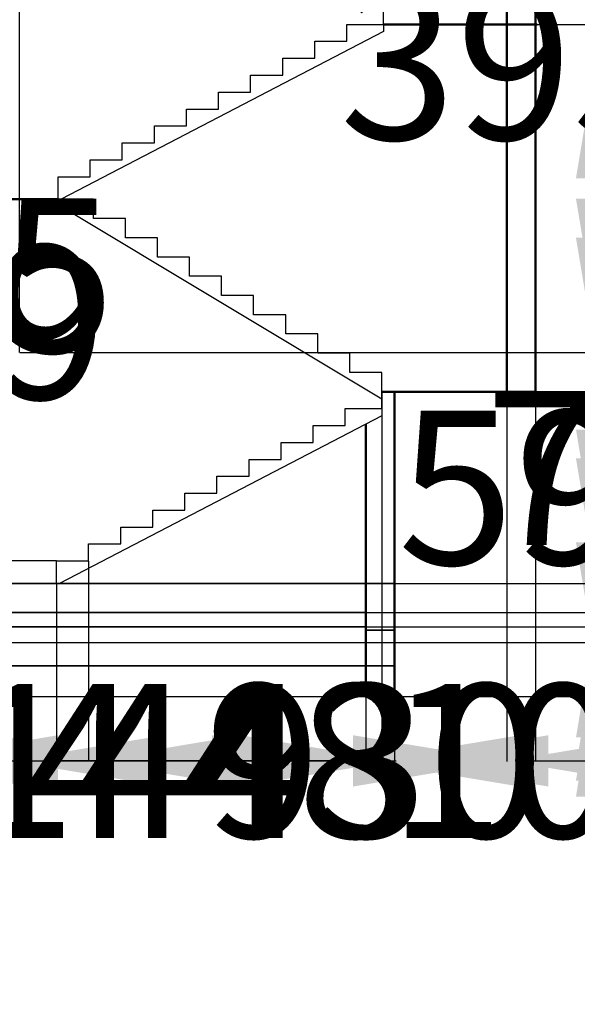
# Model space of a CAD drawing. Units: inches. Extents: x 131 to 858, y -65 to 554.
# Tile 2 of 4: x 431 to 605, y -65 to 242. Entities that reach past the tile are written whole.
import ezdxf

# ---------------------------------------------------------------- set-up
doc = ezdxf.new("R2010")
doc.units = ezdxf.units.IN
doc.header["$MEASUREMENT"] = 0
for name, color, linetype, lineweight in [('A-ANNO-DIMS', 2, 'Continuous', 18), ('A-FLOR-STRS', 3, 'Continuous', 25), ('A-SECT', 7, 'Continuous', 50), ('S-FNDN', 1, 'Continuous', 35)]:
    doc.layers.add(name, color=color, linetype=linetype, lineweight=lineweight)
doc.styles.get("Standard").update_dxf_attribs({"font": 'arial.ttf'})
doc.dimstyles.get("Standard").update_dxf_attribs({"dimtxt": 48, "dimasz": 48, "dimexe": 0.18, "dimexo": 0.0625, "dimgap": 0.09, "dimtad": 0, "dimtih": 1, "dimtoh": 1, "dimdec": 0, "dimrnd": 72, "dimzin": 0, "dimdsep": 46, "dimlunit": 3, "dimtxsty": 'Standard', "dimcen": 0.09, "dimadec": 0, "dimazin": 0, "dimtfac": 1, "dimtdec": 0, "dimtofl": 0, "dimtmove": 0, "dimatfit": 3, "dimfxl": 1, "dimtolj": 1, "dimtzin": 0, "dimarcsym": 0})

# ---------------------------------------------------------------- blocks, each defined once
blk = doc.blocks.new('*D8')
at = {"layer": 'A-ANNO-DIMS', "color": 0, "lineweight": -2, "transparency": 16777216}
for p, q in [((334.01, 66.49), (334.01, 11.06)), ((338.01, 66.49), (338.01, 11.06)), ((286.01, 11.24), (238.01, 11.24)), ((386.01, 11.24), (434.01, 11.24))]:
    blk.add_line(p, q, dxfattribs=at)
at = {"layer": 'A-ANNO-DIMS', "color": 0, "transparency": 16777216}
for points in [[(286.01, 19.24), (286.01, 3.24), (334.01, 11.24)], [(386.01, 19.24), (386.01, 3.24), (338.01, 11.24)]]:
    blk.add_solid(points, dxfattribs=at)
at = {"layer": 'Defpoints', "color": 0, "transparency": 16777216}
for p in [(334.01, 66.55), (338.01, 66.55), (338.01, 11.24)]:
    blk.add_point(p, dxfattribs=at)
at = {"layer": 'A-ANNO-DIMS', "color": 0, "transparency": 16777216, "insert": (450.7, 11.24), "char_height": 48, "attachment_point": 5}
blk.add_mtext('\\A1;4', dxfattribs=at)
blk = doc.blocks.new('*D9')
at = {"layer": 'A-ANNO-DIMS', "color": 0, "lineweight": -2, "transparency": 16777216}
for p, q in [((338.01, 66.49), (338.01, 11.06)), ((386.01, 31.27), (386.01, 11.06)), ((290.01, 11.24), (242.01, 11.24)), ((434.01, 11.24), (482.01, 11.24))]:
    blk.add_line(p, q, dxfattribs=at)
at = {"layer": 'A-ANNO-DIMS', "color": 0, "transparency": 16777216}
for points in [[(290.01, 19.24), (290.01, 3.24), (338.01, 11.24)], [(434.01, 19.24), (434.01, 3.24), (386.01, 11.24)]]:
    blk.add_solid(points, dxfattribs=at)
at = {"layer": 'Defpoints', "color": 0, "transparency": 16777216}
for p in [(338.01, 66.55), (386.01, 31.34), (386.01, 11.24)]:
    blk.add_point(p, dxfattribs=at)
at = {"layer": 'A-ANNO-DIMS', "color": 0, "transparency": 16777216, "insert": (517.5, 11.24), "char_height": 48, "attachment_point": 5}
blk.add_mtext('\\A1;48', dxfattribs=at)
blk = doc.blocks.new('*D10')
at = {"layer": 'A-ANNO-DIMS', "color": 0, "lineweight": -2, "transparency": 16777216}
for p, q in [((386.01, 31.27), (386.01, 11.06)), ((395.01, 31.27), (395.01, 11.06)), ((338.01, 11.24), (290.01, 11.24)), ((443.01, 11.24), (491.01, 11.24))]:
    blk.add_line(p, q, dxfattribs=at)
at = {"layer": 'A-ANNO-DIMS', "color": 0, "transparency": 16777216}
for points in [[(338.01, 19.24), (338.01, 3.24), (386.01, 11.24)], [(443.01, 19.24), (443.01, 3.24), (395.01, 11.24)]]:
    blk.add_solid(points, dxfattribs=at)
at = {"layer": 'Defpoints', "color": 0, "transparency": 16777216}
for p in [(386.01, 31.34), (395.01, 31.34), (395.01, 11.24)]:
    blk.add_point(p, dxfattribs=at)
at = {"layer": 'A-ANNO-DIMS', "color": 0, "transparency": 16777216, "insert": (506.89, 11.24), "char_height": 48, "attachment_point": 5}
blk.add_mtext('\\A1;9', dxfattribs=at)
blk = doc.blocks.new('*D11')
at = {"layer": 'A-ANNO-DIMS', "color": 0, "lineweight": -2, "transparency": 16777216}
for p, q in [((395.014446, 31.273524), (395.014446, 11.056024)), ((539.014446, 31.273524), (539.014446, 11.056024)), ((347.014446, 11.236024), (299.014446, 11.236024)), ((587.014446, 11.236024), (635.014446, 11.236024))]:
    blk.add_line(p, q, dxfattribs=at)
at = {"layer": 'A-ANNO-DIMS', "color": 0, "transparency": 16777216}
for points in [[(347.014446, 19.236024), (347.014446, 3.236024), (395.014446, 11.236024)], [(587.014446, 19.236024), (587.014446, 3.236024), (539.014446, 11.236024)]]:
    blk.add_solid(points, dxfattribs=at)
at = {"layer": 'Defpoints', "color": 0, "transparency": 16777216}
for p in [(395.014446, 31.336024), (539.014446, 31.336024), (539.014446, 11.236024)]:
    blk.add_point(p, dxfattribs=at)
at = {"layer": 'A-ANNO-DIMS', "color": 0, "transparency": 16777216, "insert": (467.014446, 11.236024), "char_height": 48, "attachment_point": 5}
blk.add_mtext('\\A1;144', dxfattribs=at)
blk = doc.blocks.new('*D12')
at = {"layer": 'A-ANNO-DIMS', "color": 0, "lineweight": -2, "transparency": 16777216}
for p, q in [((539.01, 31.27), (539.01, 11.06)), ((548.01, 31.27), (548.01, 11.06)), ((491.01, 11.24), (443.01, 11.24)), ((596.01, 11.24), (644.01, 11.24))]:
    blk.add_line(p, q, dxfattribs=at)
at = {"layer": 'A-ANNO-DIMS', "color": 0, "transparency": 16777216}
for points in [[(491.01, 19.24), (491.01, 3.24), (539.01, 11.24)], [(596.01, 19.24), (596.01, 3.24), (548.01, 11.24)]]:
    blk.add_solid(points, dxfattribs=at)
at = {"layer": 'Defpoints', "color": 0, "transparency": 16777216}
for p in [(539.01, 31.34), (548.01, 31.34), (548.01, 11.24)]:
    blk.add_point(p, dxfattribs=at)
at = {"layer": 'A-ANNO-DIMS', "color": 0, "transparency": 16777216, "insert": (659.89, 11.24), "char_height": 48, "attachment_point": 5}
blk.add_mtext('\\A1;9', dxfattribs=at)
blk = doc.blocks.new('*D13')
at = {"layer": 'A-ANNO-DIMS', "color": 0, "lineweight": -2, "transparency": 16777216}
for p, q in [((592.04, 126.29), (592.04, 11.06)), ((548.01, 31.27), (548.01, 11.06)), ((500.01, 11.24), (452.01, 11.24)), ((640.04, 11.24), (688.04, 11.24))]:
    blk.add_line(p, q, dxfattribs=at)
at = {"layer": 'A-ANNO-DIMS', "color": 0, "transparency": 16777216}
for points in [[(500.01, 19.24), (500.01, 3.24), (548.01, 11.24)], [(640.04, 19.24), (640.04, 3.24), (592.04, 11.24)]]:
    blk.add_solid(points, dxfattribs=at)
at = {"layer": 'Defpoints', "color": 0, "transparency": 16777216}
for p in [(592.04, 126.36), (548.01, 31.34), (592.04, 11.24)]:
    blk.add_point(p, dxfattribs=at)
at = {"layer": 'A-ANNO-DIMS', "color": 0, "transparency": 16777216, "insert": (770.09, 11.24), "char_height": 48, "attachment_point": 5}
blk.add_mtext('\\A1;44.03', dxfattribs=at)
blk = doc.blocks.new('*D14')
at = {"layer": 'A-ANNO-DIMS', "color": 0, "lineweight": -2, "transparency": 16777216}
for p, q in [((592.11, 426.55), (612.82, 426.55)), ((612.64, 378.55), (612.64, 253.56)), ((612.64, 79.34), (612.64, 204.33)), ((233.08, 31.34), (612.82, 31.34))]:
    blk.add_line(p, q, dxfattribs=at)
at = {"layer": 'A-ANNO-DIMS', "color": 0, "transparency": 16777216}
for points in [[(604.64, 378.55), (620.64, 378.55), (612.64, 426.55)], [(604.64, 79.34), (620.64, 79.34), (612.64, 31.34)]]:
    blk.add_solid(points, dxfattribs=at)
at = {"layer": 'Defpoints', "color": 0, "transparency": 16777216}
for p in [(592.04, 426.55), (612.64, 426.55), (233.01, 31.34)]:
    blk.add_point(p, dxfattribs=at)
at = {"layer": 'A-ANNO-DIMS', "color": 0, "transparency": 16777216, "insert": (612.64, 228.94), "char_height": 48, "attachment_point": 5}
blk.add_mtext('\\A1;395.2', dxfattribs=at)
blk = doc.blocks.new('*D15')
at = {"layer": 'A-ANNO-DIMS', "color": 0, "lineweight": -2, "transparency": 16777216}
for p, q in [((212.91, 114.55), (212.91, 162.55)), ((212.91, 162.55), (260.91, 162.55)), ((385.95, 66.55), (212.73, 66.55)), ((385.95, 31.34), (212.73, 31.34)), ((212.91, -16.66), (212.91, -64.66))]:
    blk.add_line(p, q, dxfattribs=at)
at = {"layer": 'A-ANNO-DIMS', "color": 0, "transparency": 16777216}
for points in [[(204.91, 114.55), (220.91, 114.55), (212.91, 66.55)], [(204.91, -16.66), (220.91, -16.66), (212.91, 31.34)]]:
    blk.add_solid(points, dxfattribs=at)
at = {"layer": 'Defpoints', "color": 0, "transparency": 16777216}
for p in [(212.91, 66.55), (386.01, 66.55), (386.01, 31.34)]:
    blk.add_point(p, dxfattribs=at)
at = {"layer": 'A-ANNO-DIMS', "color": 0, "transparency": 16777216, "insert": (360.8, 162.55), "char_height": 48, "attachment_point": 5}
blk.add_mtext('\\A1;35.215', dxfattribs=at)
blk = doc.blocks.new('*D17')
at = {"layer": 'A-ANNO-DIMS', "color": 0, "lineweight": -2, "transparency": 16777216}
for p, q in [((212.91, 100.02), (212.91, 148.02)), ((212.91, 148.02), (260.91, 148.02)), ((232.95, 52.02), (212.73, 52.02)), ((232.95, 40.9), (212.73, 40.9)), ((212.91, -7.1), (212.91, -55.1))]:
    blk.add_line(p, q, dxfattribs=at)
at = {"layer": 'A-ANNO-DIMS', "color": 0, "transparency": 16777216}
for points in [[(204.91, 100.02), (220.91, 100.02), (212.91, 52.02)], [(204.91, -7.1), (220.91, -7.1), (212.91, 40.9)]]:
    blk.add_solid(points, dxfattribs=at)
at = {"layer": 'Defpoints', "color": 0, "transparency": 16777216}
for p in [(212.91, 52.02), (233.01, 52.02), (233.01, 40.9)]:
    blk.add_point(p, dxfattribs=at)
at = {"layer": 'A-ANNO-DIMS', "color": 0, "transparency": 16777216, "insert": (358.43, 148.02), "char_height": 48, "attachment_point": 5}
blk.add_mtext('\\A1;11.119', dxfattribs=at)
blk = doc.blocks.new('*D19')
at = {"layer": 'A-ANNO-DIMS', "color": 0, "lineweight": -2, "transparency": 16777216}
for p, q in [((612.64, 105.55), (612.64, 153.55)), ((612.64, 153.55), (660.64, 153.55)), ((242.08, 57.55), (612.82, 57.55)), ((242.08, 53.09), (612.82, 53.09)), ((612.64, 5.09), (612.64, -42.91))]:
    blk.add_line(p, q, dxfattribs=at)
at = {"layer": 'A-ANNO-DIMS', "color": 0, "transparency": 16777216}
for points in [[(604.64, 105.55), (620.64, 105.55), (612.64, 57.55)], [(604.64, 5.09), (620.64, 5.09), (612.64, 53.09)]]:
    blk.add_solid(points, dxfattribs=at)
at = {"layer": 'Defpoints', "color": 0, "transparency": 16777216}
for p in [(242.01, 57.55), (612.64, 57.55), (242.01, 53.09)]:
    blk.add_point(p, dxfattribs=at)
at = {"layer": 'A-ANNO-DIMS', "color": 0, "transparency": 16777216, "insert": (742.86, 153.55), "char_height": 48, "attachment_point": 5}
blk.add_mtext('\\A1;4.465', dxfattribs=at)
blk = doc.blocks.new('*D20')
at = {"layer": 'A-ANNO-DIMS', "color": 0, "lineweight": -2, "transparency": 16777216}
for p, q in [((612.64, 114.55), (612.64, 162.55)), ((612.64, 162.55), (660.64, 162.55)), ((242.08, 66.55), (612.82, 66.55)), ((242.08, 57.55), (612.82, 57.55)), ((612.64, 9.55), (612.64, -38.45))]:
    blk.add_line(p, q, dxfattribs=at)
at = {"layer": 'A-ANNO-DIMS', "color": 0, "transparency": 16777216}
for points in [[(604.64, 114.55), (620.64, 114.55), (612.64, 66.55)], [(604.64, 9.55), (620.64, 9.55), (612.64, 57.55)]]:
    blk.add_solid(points, dxfattribs=at)
at = {"layer": 'Defpoints', "color": 0, "transparency": 16777216}
for p in [(242.01, 66.55), (612.64, 66.55), (242.01, 57.55)]:
    blk.add_point(p, dxfattribs=at)
at = {"layer": 'A-ANNO-DIMS', "color": 0, "transparency": 16777216, "insert": (676.51, 162.55), "char_height": 48, "attachment_point": 5}
blk.add_mtext('\\A1;9', dxfattribs=at)
blk = doc.blocks.new('*D22')
at = {"layer": 'A-ANNO-DIMS', "color": 0, "lineweight": -2, "transparency": 16777216}
for p, q in [((612.64, 114.55), (612.64, 162.55)), ((612.64, 162.55), (660.64, 162.55)), ((395.08, 66.55), (612.82, 66.55)), ((395.08, 48.13), (612.82, 48.13)), ((612.64, 0.13), (612.64, -47.87))]:
    blk.add_line(p, q, dxfattribs=at)
at = {"layer": 'A-ANNO-DIMS', "color": 0, "transparency": 16777216}
for points in [[(604.64, 114.55), (620.64, 114.55), (612.64, 66.55)], [(604.64, 0.13), (620.64, 0.13), (612.64, 48.13)]]:
    blk.add_solid(points, dxfattribs=at)
at = {"layer": 'Defpoints', "color": 0, "transparency": 16777216}
for p in [(395.01, 66.55), (612.64, 66.55), (395.01, 48.13)]:
    blk.add_point(p, dxfattribs=at)
at = {"layer": 'A-ANNO-DIMS', "color": 0, "transparency": 16777216, "insert": (758.11, 162.55), "char_height": 48, "attachment_point": 5}
blk.add_mtext('\\A1;18.417', dxfattribs=at)
blk = doc.blocks.new('*D32')
at = {"layer": 'A-ANNO-DIMS', "color": 0, "lineweight": -2, "transparency": 16777216}
for p, q in [((347.01, 446.65), (299.01, 446.65)), ((395.01, 138.61), (395.01, 446.83)), ((431.01, 138.61), (431.01, 446.83)), ((479.01, 446.65), (527.01, 446.65))]:
    blk.add_line(p, q, dxfattribs=at)
at = {"layer": 'A-ANNO-DIMS', "color": 0, "transparency": 16777216}
for points in [[(347.01, 454.65), (347.01, 438.65), (395.01, 446.65)], [(479.01, 454.65), (479.01, 438.65), (431.01, 446.65)]]:
    blk.add_solid(points, dxfattribs=at)
at = {"layer": 'Defpoints', "color": 0, "transparency": 16777216}
for p in [(431.01, 446.65), (395.01, 138.55), (431.01, 138.55)]:
    blk.add_point(p, dxfattribs=at)
at = {"layer": 'A-ANNO-DIMS', "color": 0, "transparency": 16777216, "insert": (561.45, 446.65), "char_height": 48, "attachment_point": 5}
blk.add_mtext('\\A1;36', dxfattribs=at)
blk = doc.blocks.new('*D33')
at = {"layer": 'A-ANNO-DIMS', "color": 0, "lineweight": -2, "transparency": 16777216}
for p, q in [((612.639956, 186.551418), (612.639956, 234.551418)), ((431.076946, 138.551418), (612.819956, 138.551418)), ((431.076946, 66.551418), (612.819956, 66.551418)), ((612.639956, 18.551418), (612.639956, -29.448582))]:
    blk.add_line(p, q, dxfattribs=at)
at = {"layer": 'A-ANNO-DIMS', "color": 0, "transparency": 16777216}
for points in [[(604.639956, 186.551418), (620.639956, 186.551418), (612.639956, 138.551418)], [(604.639956, 18.551418), (620.639956, 18.551418), (612.639956, 66.551418)]]:
    blk.add_solid(points, dxfattribs=at)
at = {"layer": 'Defpoints', "color": 0, "transparency": 16777216}
for p in [(431.014446, 138.551418), (612.639956, 138.551418), (431.014446, 66.551418)]:
    blk.add_point(p, dxfattribs=at)
at = {"layer": 'A-ANNO-DIMS', "color": 0, "transparency": 16777216, "insert": (612.639956, 102.551418), "char_height": 48, "attachment_point": 5}
blk.add_mtext('\\A1;72', dxfattribs=at)
blk = doc.blocks.new('*D34')
at = {"layer": 'A-ANNO-DIMS', "color": 0, "lineweight": -2, "transparency": 16777216}
for p, q in [((398.01, 66.49), (398.01, 11.06)), ((428.01, 66.49), (428.01, 11.06)), ((350.01, 11.24), (302.01, 11.24)), ((476.01, 11.24), (524.01, 11.24))]:
    blk.add_line(p, q, dxfattribs=at)
at = {"layer": 'A-ANNO-DIMS', "color": 0, "transparency": 16777216}
for points in [[(350.01, 19.24), (350.01, 3.24), (398.01, 11.24)], [(476.01, 19.24), (476.01, 3.24), (428.01, 11.24)]]:
    blk.add_solid(points, dxfattribs=at)
at = {"layer": 'Defpoints', "color": 0, "transparency": 16777216}
for p in [(398.01, 66.55), (428.01, 66.55), (428.01, 11.24)]:
    blk.add_point(p, dxfattribs=at)
at = {"layer": 'A-ANNO-DIMS', "color": 0, "transparency": 16777216, "insert": (558.39, 11.24), "char_height": 48, "attachment_point": 5}
blk.add_mtext('\\A1;30', dxfattribs=at)
blk = doc.blocks.new('*D36')
at = {"layer": 'A-ANNO-DIMS', "color": 0, "lineweight": -2, "transparency": 16777216}
for p, q in [((452.53, 73.54), (452.53, 11.06)), ((442.52, 66.49), (442.52, 11.06)), ((394.52, 11.24), (346.52, 11.24)), ((500.53, 11.24), (548.53, 11.24))]:
    blk.add_line(p, q, dxfattribs=at)
at = {"layer": 'A-ANNO-DIMS', "color": 0, "transparency": 16777216}
for points in [[(394.52, 19.24), (394.52, 3.24), (442.52, 11.24)], [(500.53, 19.24), (500.53, 3.24), (452.53, 11.24)]]:
    blk.add_solid(points, dxfattribs=at)
at = {"layer": 'Defpoints', "color": 0, "transparency": 16777216}
for p in [(452.53, 73.6), (442.52, 66.55), (452.53, 11.24)]:
    blk.add_point(p, dxfattribs=at)
at = {"layer": 'A-ANNO-DIMS', "color": 0, "transparency": 16777216, "insert": (646, 11.24), "char_height": 48, "attachment_point": 5}
blk.add_mtext('\\A1;10.013', dxfattribs=at)
blk = doc.blocks.new('*D37')
at = {"layer": 'A-ANNO-DIMS', "color": 0, "lineweight": -2, "transparency": 16777216}
for p, q in [((544.04, 126.29), (544.04, 11.06)), ((452.53, 73.54), (452.53, 11.06)), ((404.53, 11.24), (356.53, 11.24)), ((592.04, 11.24), (640.04, 11.24))]:
    blk.add_line(p, q, dxfattribs=at)
at = {"layer": 'A-ANNO-DIMS', "color": 0, "transparency": 16777216}
for points in [[(404.53, 19.24), (404.53, 3.24), (452.53, 11.24)], [(592.04, 19.24), (592.04, 3.24), (544.04, 11.24)]]:
    blk.add_solid(points, dxfattribs=at)
at = {"layer": 'Defpoints', "color": 0, "transparency": 16777216}
for p in [(544.04, 126.36), (452.53, 73.6), (544.04, 11.24)]:
    blk.add_point(p, dxfattribs=at)
at = {"layer": 'A-ANNO-DIMS', "color": 0, "transparency": 16777216, "insert": (716.49, 11.24), "char_height": 48, "attachment_point": 5}
blk.add_mtext('\\A1;91.51', dxfattribs=at)
blk = doc.blocks.new('*D38')
at = {"layer": 'A-ANNO-DIMS', "color": 0, "lineweight": -2, "transparency": 16777216}
for p, q in [((544.04, 126.29), (544.04, 11.06)), ((583.04, 126.29), (583.04, 11.06)), ((496.04, 11.24), (448.04, 11.24)), ((631.04, 11.24), (679.04, 11.24))]:
    blk.add_line(p, q, dxfattribs=at)
at = {"layer": 'A-ANNO-DIMS', "color": 0, "transparency": 16777216}
for points in [[(496.04, 19.24), (496.04, 3.24), (544.04, 11.24)], [(631.04, 19.24), (631.04, 3.24), (583.04, 11.24)]]:
    blk.add_solid(points, dxfattribs=at)
at = {"layer": 'Defpoints', "color": 0, "transparency": 16777216}
for p in [(544.04, 126.36), (583.04, 126.36), (583.04, 11.24)]:
    blk.add_point(p, dxfattribs=at)
at = {"layer": 'A-ANNO-DIMS', "color": 0, "transparency": 16777216, "insert": (713.55, 11.24), "char_height": 48, "attachment_point": 5}
blk.add_mtext('\\A1;39', dxfattribs=at)
blk = doc.blocks.new('*D39')
at = {"layer": 'A-ANNO-DIMS', "color": 0, "lineweight": -2, "transparency": 16777216}
for p, q in [((583.04, 126.29), (583.04, 11.06)), ((592.04, 126.29), (592.04, 11.06)), ((535.04, 11.24), (487.04, 11.24)), ((640.04, 11.24), (688.04, 11.24))]:
    blk.add_line(p, q, dxfattribs=at)
at = {"layer": 'A-ANNO-DIMS', "color": 0, "transparency": 16777216}
for points in [[(535.04, 19.24), (535.04, 3.24), (583.04, 11.24)], [(640.04, 19.24), (640.04, 3.24), (592.04, 11.24)]]:
    blk.add_solid(points, dxfattribs=at)
at = {"layer": 'Defpoints', "color": 0, "transparency": 16777216}
for p in [(583.04, 126.36), (592.04, 126.36), (592.04, 11.24)]:
    blk.add_point(p, dxfattribs=at)
at = {"layer": 'A-ANNO-DIMS', "color": 0, "transparency": 16777216, "insert": (703.92, 11.24), "char_height": 48, "attachment_point": 5}
blk.add_mtext('\\A1;9', dxfattribs=at)
blk = doc.blocks.new('*D40')
at = {"layer": 'A-ANNO-DIMS', "color": 0, "lineweight": -2, "transparency": 16777216}
for p, q in [((212.91, 121.6), (212.91, 169.6)), ((212.91, 169.6), (260.91, 169.6)), ((442.46, 73.6), (212.73, 73.6)), ((442.46, 66.55), (212.73, 66.55)), ((212.91, 18.55), (212.91, -29.45))]:
    blk.add_line(p, q, dxfattribs=at)
at = {"layer": 'A-ANNO-DIMS', "color": 0, "transparency": 16777216}
for points in [[(204.91, 121.6), (220.91, 121.6), (212.91, 73.6)], [(204.91, 18.55), (220.91, 18.55), (212.91, 66.55)]]:
    blk.add_solid(points, dxfattribs=at)
at = {"layer": 'Defpoints', "color": 0, "transparency": 16777216}
for p in [(212.91, 73.6), (442.52, 73.6), (442.52, 66.55)]:
    blk.add_point(p, dxfattribs=at)
at = {"layer": 'A-ANNO-DIMS', "color": 0, "transparency": 16777216, "insert": (323.33, 169.6), "char_height": 48, "attachment_point": 5}
blk.add_mtext('\\A1;7.05', dxfattribs=at)
blk = doc.blocks.new('*D41')
at = {"layer": 'A-ANNO-DIMS', "color": 0, "lineweight": -2, "transparency": 16777216}
for p, q in [((612.64, 174.36), (612.64, 222.36)), ((592.11, 126.36), (612.82, 126.36)), ((548.08, 66.55), (612.82, 66.55)), ((612.64, 18.55), (612.64, -29.45))]:
    blk.add_line(p, q, dxfattribs=at)
at = {"layer": 'A-ANNO-DIMS', "color": 0, "transparency": 16777216}
for points in [[(604.64, 174.36), (620.64, 174.36), (612.64, 126.36)], [(604.64, 18.55), (620.64, 18.55), (612.64, 66.55)]]:
    blk.add_solid(points, dxfattribs=at)
at = {"layer": 'Defpoints', "color": 0, "transparency": 16777216}
for p in [(592.04, 126.36), (612.64, 126.36), (548.01, 66.55)]:
    blk.add_point(p, dxfattribs=at)
at = {"layer": 'A-ANNO-DIMS', "color": 0, "transparency": 16777216, "insert": (612.64, 96.45), "char_height": 48, "attachment_point": 5}
blk.add_mtext('\\A1;59.8', dxfattribs=at)
blk = doc.blocks.new('*D42')
at = {"layer": 'A-ANNO-DIMS', "color": 0, "lineweight": -2, "transparency": 16777216}
for p, q in [((612.64, 240.89), (612.64, 288.89)), ((612.64, 288.89), (660.64, 288.89)), ((592.6, 240.89), (612.82, 240.89)), ((612.64, 174.36), (612.64, 192.89)), ((592.11, 126.36), (612.82, 126.36))]:
    blk.add_line(p, q, dxfattribs=at)
at = {"layer": 'A-ANNO-DIMS', "color": 0, "transparency": 16777216}
for points in [[(604.64, 192.89), (620.64, 192.89), (612.64, 240.89)], [(604.64, 174.36), (620.64, 174.36), (612.64, 126.36)]]:
    blk.add_solid(points, dxfattribs=at)
at = {"layer": 'Defpoints', "color": 0, "transparency": 16777216}
for p in [(592.54, 240.89), (612.64, 240.89), (592.04, 126.36)]:
    blk.add_point(p, dxfattribs=at)
at = {"layer": 'A-ANNO-DIMS', "color": 0, "transparency": 16777216, "insert": (758.11, 288.89), "char_height": 48, "attachment_point": 5}
blk.add_mtext('\\A1;114.53', dxfattribs=at)
blk = doc.blocks.new('*D43')
at = {"layer": 'A-ANNO-DIMS', "color": 0, "lineweight": -2, "transparency": 16777216}
for p, q in [((612.639956, 354.551418), (612.639956, 402.551418)), ((443.076946, 306.551418), (612.819956, 306.551418)), ((592.602456, 240.886672), (612.819956, 240.886672)), ((612.639956, 192.886672), (612.639956, 144.886672))]:
    blk.add_line(p, q, dxfattribs=at)
at = {"layer": 'A-ANNO-DIMS', "color": 0, "transparency": 16777216}
for points in [[(604.639956, 354.551418), (620.639956, 354.551418), (612.639956, 306.551418)], [(604.639956, 192.886672), (620.639956, 192.886672), (612.639956, 240.886672)]]:
    blk.add_solid(points, dxfattribs=at)
at = {"layer": 'Defpoints', "color": 0, "transparency": 16777216}
for p in [(443.014446, 306.551418), (612.639956, 306.551418), (592.539956, 240.886672)]:
    blk.add_point(p, dxfattribs=at)
at = {"layer": 'A-ANNO-DIMS', "color": 0, "transparency": 16777216, "insert": (612.639956, 273.719045), "char_height": 48, "attachment_point": 5}
blk.add_mtext('\\A1;65.66', dxfattribs=at)

msp = doc.modelspace()

# ---------------------------------------------------------------- linework, layer by layer
at = {"layer": 'A-FLOR-STRS'}
for p, q in [((544.54, 240.8867), (544.54, 246.1622)), ((533.1288, 235.6112), (533.1288, 240.8867)), ((533.1288, 240.8867), (543.1415, 240.8867)), ((543.1415, 240.8867), (544.54, 240.8867)), ((544.54, 240.8867), (544.54, 238.6328)), ((544.54, 238.6328), (443.9366, 186.3568)), ((523.1161, 230.3356), (523.1161, 235.6112)), ((523.1161, 235.6112), (533.1288, 235.6112)), ((513.1034, 225.0601), (513.1034, 230.3356)), ((513.1034, 230.3356), (523.1161, 230.3356)), ((503.0907, 219.7846), (503.0907, 225.0601)), ((503.0907, 225.0601), (513.1034, 225.0601)), ((493.078, 214.5091), (493.078, 219.7846)), ((493.078, 219.7846), (503.0907, 219.7846)), ((483.0653, 209.2336), (483.0653, 214.5091)), ((483.0653, 214.5091), (493.078, 214.5091)), ((473.0526, 203.9581), (473.0526, 209.2336)), ((473.0526, 209.2336), (483.0653, 209.2336)), ((473.0526, 203.9581), (473.0526, 209.2336)), ((473.0526, 209.2336), (483.0653, 209.2336)), ((463.0399, 198.6825), (463.0399, 203.9581)), ((463.0399, 203.9581), (473.0526, 203.9581)), ((453.0272, 193.407), (453.0272, 198.6825)), ((453.0272, 198.6825), (463.0399, 198.6825)), ((453.0272, 193.407), (453.0272, 198.6825)), ((453.0272, 198.6825), (463.0399, 198.6825)), ((443.0144, 186.3568), (443.0144, 193.407)), ((443.0144, 193.407), (453.0272, 193.407)), ((443.0144, 184.6418), (443.0144, 186.3568)), ((443.0144, 186.3568), (444.0434, 186.3568)), ((443.9366, 186.3568), (443.0144, 186.3568)), ((544.0434, 124.0244), (443.0144, 184.6418)), ((454.0434, 186.3568), (444.0434, 186.3568)), ((454.0434, 180.3568), (454.0434, 186.3568)), ((454.0434, 186.3568), (454.0434, 186.3568)), ((464.0434, 180.3568), (454.0434, 180.3568)), ((464.0434, 174.3568), (464.0434, 180.3568)), ((464.0434, 180.3568), (464.0434, 180.3568)), ((474.0434, 174.3568), (464.0434, 174.3568)), ((474.0434, 168.3568), (474.0434, 174.3568)), ((474.0434, 174.3568), (474.0434, 174.3568)), ((484.0434, 168.3568), (474.0434, 168.3568)), ((484.0434, 162.3568), (484.0434, 168.3568)), ((484.0434, 168.3568), (484.0434, 168.3568)), ((494.0434, 162.3568), (484.0434, 162.3568)), ((494.0434, 156.3568), (494.0434, 162.3568)), ((494.0434, 162.3568), (494.0434, 162.3568)), ((504.0434, 156.3568), (494.0434, 156.3568)), ((504.0434, 150.3568), (504.0434, 156.3568)), ((504.0434, 156.3568), (504.0434, 156.3568)), ((514.0434, 150.3568), (504.0434, 150.3568)), ((514.0434, 144.3568), (514.0434, 150.3568)), ((514.0434, 150.3568), (514.0434, 150.3568)), ((524.0434, 144.3568), (514.0434, 144.3568)), ((524.0434, 138.3568), (524.0434, 144.3568)), ((524.0434, 144.3568), (524.0434, 144.3568)), ((534.0434, 138.3568), (524.0434, 138.3568)), ((534.0434, 132.3568), (534.0434, 138.3568)), ((534.0434, 138.3568), (534.0434, 138.3568)), ((544.0434, 132.3568), (534.0434, 132.3568)), ((544.0434, 126.3568), (544.0434, 132.3568)), ((544.0434, 132.3568), (544.0434, 132.3568)), ((544.0434, 121.0813), (544.0434, 126.3568)), ((544.0434, 126.3568), (554.0561, 126.3568)), ((554.0561, 126.3568), (555.4546, 126.3568)), ((532.6323, 115.8058), (532.6323, 121.0813)), ((532.6323, 121.0813), (542.645, 121.0813)), ((542.645, 121.0813), (544.0434, 121.0813)), ((544.0434, 121.0813), (544.0434, 118.8274)), ((544.0434, 118.8274), (443.4401, 66.5514)), ((522.6196, 110.5303), (522.6196, 115.8058)), ((522.6196, 115.8058), (532.6323, 115.8058)), ((512.6069, 105.2547), (512.6069, 110.5303)), ((512.6069, 110.5303), (522.6196, 110.5303)), ((502.5942, 99.9792), (502.5942, 105.2547)), ((502.5942, 105.2547), (512.6069, 105.2547)), ((492.5815, 94.7037), (492.5815, 99.9792)), ((492.5815, 99.9792), (502.5942, 99.9792)), ((482.5688, 89.4282), (482.5688, 94.7037)), ((482.5688, 94.7037), (492.5815, 94.7037)), ((472.5561, 84.1527), (472.5561, 89.4282)), ((472.5561, 89.4282), (482.5688, 89.4282)), ((472.5561, 84.1527), (472.5561, 89.4282)), ((472.5561, 89.4282), (482.5688, 89.4282)), ((462.5433, 78.8772), (462.5433, 84.1527)), ((462.5433, 84.1527), (472.5561, 84.1527)), ((452.5306, 73.6016), (452.5306, 78.8772)), ((452.5306, 78.8772), (462.5433, 78.8772)), ((452.5306, 73.6016), (452.5306, 78.8772)), ((452.5306, 78.8772), (462.5433, 78.8772)), ((442.5179, 66.5514), (442.5179, 73.6016)), ((442.5179, 73.6016), (452.5306, 73.6016))]:
    msp.add_line(p, q, dxfattribs=at)
at = {"layer": 'A-SECT'}
for p, q in [((583.0434, 126.3568), (583.0434, 426.5514)), ((592.0434, 126.3568), (592.0434, 426.5514)), ((544.54, 240.8867), (592.54, 240.8867)), ((395.0144, 186.3568), (443.0144, 186.3568)), ((544.0434, 126.3568), (592.0434, 126.3568)), ((548.0144, 126.5514), (548.0144, 31.336)), ((539.0144, 66.5514), (539.0144, 116.2142)), ((539.0144, 116.2142), (539.0144, 31.336))]:
    msp.add_line(p, q, dxfattribs=at)
at = {"layer": 'S-FNDN'}
for p, q in [((442.5179, 66.5514), (386.0144, 66.5514)), ((395.0144, 66.5514), (548.0144, 66.5514)), ((443.4401, 66.5514), (442.5179, 66.5514)), ((539.0144, 66.5514), (548.0144, 66.5514)), ((548.0144, 66.5514), (539.0144, 66.5514)), ((539.0144, 66.5514), (539.0144, 57.5514)), ((548.0144, 66.5514), (539.0144, 66.5514)), ((548.0144, 66.5514), (548.0144, 57.5514)), ((395.0144, 57.5514), (539.0144, 57.5514)), ((395.0144, 53.0868), (539.0144, 53.0868)), ((539.0144, 52.0226), (548.0144, 52.0226)), ((539.0144, 52.0226), (548.0144, 52.0226)), ((233.0144, 40.9038), (548.0144, 40.9038)), ((539.0144, 31.336), (548.0144, 31.336))]:
    msp.add_line(p, q, dxfattribs=at)

# ---------------------------------------------------------------- dimensions: what is measured, and where the dimension line sits
at = {"layer": 'A-ANNO-DIMS'}
for base, p1, p2, override, picture, middle in [((431.0144, 446.6514), (395.0144, 138.5514), (431.0144, 138.5514), {"dimdec": 0, "dimlfac": 1, "dimrnd": 0, "dimzin": 0, "dimdsep": 46, "dimlunit": 2}, '*D32', (561.451, 446.6514)), ((544.0434, 11.236), (452.5306, 73.6016), (544.0434, 126.3568), {"dimdec": 2, "dimlfac": 1, "dimrnd": 0, "dimzin": 0, "dimdsep": 46, "dimlunit": 2}, '*D37', (716.4881, 11.236)), ((583.0434, 11.236), (544.0434, 126.3568), (583.0434, 126.3568), {"dimdec": 0, "dimlfac": 1, "dimrnd": 0, "dimzin": 0, "dimdsep": 46, "dimlunit": 2}, '*D38', (713.5454, 11.236)), ((592.0434, 11.236), (548.0144, 31.336), (592.0434, 126.3568), {"dimdec": 2, "dimlfac": 1, "dimrnd": 0, "dimzin": 0, "dimdsep": 46, "dimlunit": 2}, '*D13', (770.0871, 11.236)), ((592.0434, 11.236), (583.0434, 126.3568), (592.0434, 126.3568), {"dimdec": 0, "dimlfac": 1, "dimrnd": 0, "dimzin": 0, "dimdsep": 46, "dimlunit": 2}, '*D39', (703.9152, 11.236)), ((452.5306, 11.236), (442.5179, 66.5514), (452.5306, 73.6016), {"dimdec": 3, "dimlfac": 1, "dimrnd": 0, "dimzin": 0, "dimdsep": 46, "dimlunit": 2}, '*D36', (645.9958, 11.236)), ((338.0144, 11.236), (334.0144, 66.5514), (338.0144, 66.5514), {"dimdec": 0, "dimlfac": 1, "dimrnd": 0, "dimzin": 0, "dimdsep": 46, "dimlunit": 2}, '*D8', (450.7047, 11.236)), ((386.0144, 11.236), (338.0144, 66.5514), (386.0144, 31.336), {"dimdec": 0, "dimlfac": 1, "dimrnd": 0, "dimzin": 0, "dimdsep": 46, "dimlunit": 2}, '*D9', (517.4987, 11.236)), ((428.0144, 11.236), (398.0144, 66.5514), (428.0144, 66.5514), {"dimdec": 0, "dimlfac": 1, "dimrnd": 0, "dimzin": 0, "dimdsep": 46, "dimlunit": 2}, '*D34', (558.3855, 11.236)), ((395.0144, 11.236), (386.0144, 31.336), (395.0144, 31.336), {"dimdec": 0, "dimlfac": 1, "dimrnd": 0, "dimzin": 0, "dimdsep": 46, "dimlunit": 2}, '*D10', (506.8862, 11.236)), ((539.0144, 11.236), (395.0144, 31.336), (539.0144, 31.336), {"dimdec": 0, "dimlfac": 1, "dimrnd": 0, "dimzin": 0, "dimdsep": 46, "dimlunit": 2}, '*D11', (467.0144, 11.236)), ((548.0144, 11.236), (539.0144, 31.336), (548.0144, 31.336), {"dimdec": 0, "dimlfac": 1, "dimrnd": 0, "dimzin": 0, "dimdsep": 46, "dimlunit": 2}, '*D12', (659.8862, 11.236))]:
    dim = msp.add_linear_dim(base=base, p1=p1, p2=p2, dimstyle='Standard', override=override, dxfattribs=at)
    dim.commit()
    dim.dimension.update_dxf_attribs({"geometry": picture, "text_midpoint": middle})
for base, p1, p2, override, picture, middle in [((612.64, 426.5514), (233.0144, 31.336), (592.0434, 426.5514), {"dimdec": 1, "dimlfac": 1, "dimrnd": 0, "dimzin": 0, "dimdsep": 46, "dimlunit": 2}, '*D14', (612.64, 228.9437)), ((612.64, 306.5514), (592.54, 240.8867), (443.0144, 306.5514), {"dimdec": 2, "dimlfac": 1, "dimrnd": 0, "dimzin": 0, "dimdsep": 46, "dimlunit": 2}, '*D43', (612.64, 273.719)), ((612.64, 240.8867), (592.0434, 126.3568), (592.54, 240.8867), {"dimdec": 2, "dimlfac": 1, "dimrnd": 0, "dimzin": 0, "dimdsep": 46, "dimlunit": 2}, '*D42', (758.1051, 288.8867)), ((612.64, 138.5514), (431.0144, 66.5514), (431.0144, 138.5514), {"dimdec": 0, "dimlfac": 1, "dimrnd": 0, "dimzin": 0, "dimdsep": 46, "dimlunit": 2}, '*D33', (612.64, 102.5514)), ((612.64, 126.3568), (548.0144, 66.5514), (592.0434, 126.3568), {"dimdec": 1, "dimlfac": 1, "dimrnd": 0, "dimzin": 0, "dimdsep": 46, "dimlunit": 2}, '*D41', (612.64, 96.4541)), ((212.9144, 73.6016), (442.5179, 66.5514), (442.5179, 73.6016), {"dimdec": 2, "dimlfac": 1, "dimrnd": 0, "dimzin": 0, "dimdsep": 46, "dimlunit": 2}, '*D40', (323.3291, 169.6016)), ((212.9144, 66.5514), (386.0144, 31.336), (386.0144, 66.5514), {"dimdec": 3, "dimlfac": 1, "dimrnd": 0, "dimzin": 0, "dimdsep": 46, "dimlunit": 2}, '*D15', (360.8025, 162.5514)), ((612.64, 66.5514), (242.0144, 57.5514), (242.0144, 66.5514), {"dimdec": 0, "dimlfac": 1, "dimrnd": 0, "dimzin": 0, "dimdsep": 46, "dimlunit": 2}, '*D20', (676.5117, 162.5514)), ((612.64, 66.5514), (395.0144, 48.1342), (395.0144, 66.5514), {"dimdec": 3, "dimlfac": 1, "dimrnd": 0, "dimzin": 0, "dimdsep": 46, "dimlunit": 2}, '*D22', (758.1051, 162.5514)), ((612.64, 57.5514), (242.0144, 53.0868), (242.0144, 57.5514), {"dimdec": 3, "dimlfac": 1, "dimrnd": 0, "dimzin": 0, "dimdsep": 46, "dimlunit": 2}, '*D19', (742.8637, 153.5514)), ((212.9144, 52.0226), (233.0144, 40.9038), (233.0144, 52.0226), {"dimdec": 3, "dimlfac": 1, "dimrnd": 0, "dimzin": 0, "dimdsep": 46, "dimlunit": 2}, '*D17', (358.4287, 148.0226))]:
    dim = msp.add_linear_dim(base=base, p1=p1, p2=p2, angle=90, dimstyle='Standard', override=override, dxfattribs=at)
    dim.commit()
    dim.dimension.update_dxf_attribs({"geometry": picture, "text_midpoint": middle})

doc.saveas('drawing.dxf')
